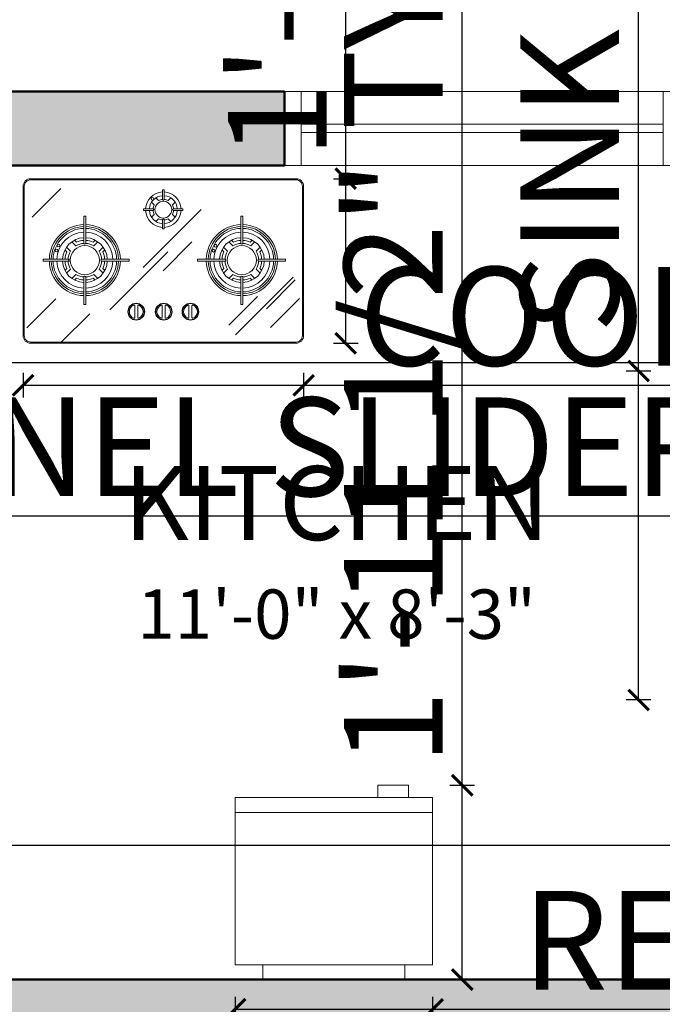
# Model space of a CAD drawing. Units: inches. Extents: x 375 to 1122, y 27 to 1069.
# Tile 152 of 155: x 819 to 897, y 872 to 991. Entities that reach past the tile are written whole.
import ezdxf

# ---------------------------------------------------------------- set-up
doc = ezdxf.new("R2010")
doc.units = ezdxf.units.IN
for name, color, linetype, lineweight in [('A-ANNO-DIMS', 2, 'Continuous', 18), ('A-AREA-IDEN', 7, 'Continuous', 18), ('A-EQPM', 55, 'Continuous', 18), ('A-FLOR-MILL', 55, 'Continuous', 25), ('A-WALL-PATT', 252, 'Continuous', 13), ('Walls', 250, 'Continuous', 50), ('Windows', 122, 'Continuous', 18)]:
    doc.layers.add(name, color=color, linetype=linetype, lineweight=lineweight)
doc.styles.get("Standard").update_dxf_attribs({"font": 'arial.ttf'})
doc.dimstyles.new('ISO-25', dxfattribs={"dimtxt": 12, "dimasz": 2.5, "dimexe": 1.5, "dimexo": 1.5, "dimtad": 1, "dimdec": 1, "dimlunit": 3, "dimtxsty": 'Standard', "dimblk": 'ARCHTICK', "dimcen": 2.5, "dimadec": 0, "dimazin": 0, "dimtfac": 1, "dimtdec": 1, "dimtmove": 0, "dimatfit": 3, "dimfxl": 1.5, "dimfxlon": 1, "dimarcsym": 0})

# ---------------------------------------------------------------- blocks, each defined once
blk = doc.blocks.new('A$C659B0DF6')
for p, q in [((17.35, 607.55), (17.35, 606.07)), ((21.05, 607.55), (17.35, 607.55)), ((21.05, 606.07), (21.05, 607.55)), ((24, 606.07), (0, 606.07)), ((0, 585.72), (0, 606.07)), ((24, 585.72), (24, 606.07)), ((24, 604.22), (0, 604.22)), ((24, 585.72), (0, 585.72)), ((3.37, 583.91), (3.37, 585.72)), ((20.63, 583.91), (20.63, 585.72)), ((3.37, 583.91), (20.63, 583.91))]:
    blk.add_line(p, q)
blk = doc.blocks.new('A$C038F079D')
for p, q in [((23.9, 336.8), (101.3, 414.2)), ((377.5, 410.6), (372.5, 410.6)), ((320.9, 202.7), (475.7, 357.5)), ((427.1, 359.8), (427.1, 354.8)), ((587.4, 339.9), (582.4, 339.9)), ((377.5, 305.6), (372.5, 305.6)), ((374.2, 193.8), (451.6, 271.2)), ((232.1, 89.3), (386.9, 244.1)), ((53.2, 224.7), (53.2, 219.7)), ((284, 224.7), (284, 219.7)), ((466, 224.7), (466, 219.7)), ((701.8, 224.7), (701.8, 219.7)), ((130.3, 173.3), (141.1, 184.1)), ((137.3, 169), (142.6, 174.2)), ((567.6, 22.2), (722.4, 177)), ((650.5, 92.2), (727.9, 169.6)), ((10.1, 41), (87.5, 118.4)), ((549.9, 47.9), (627.2, 125.3)), ((661.4, 42), (738.7, 119.3)), ((587.4, 103.7), (582.4, 103.7)), ((100.9, 1.5), (178.3, 78.9))]:
    blk.add_line(p, q)
at = {"ltscale": 0.18}
for p, q in [((372.5, 384.7), (372.5, 410.6)), ((377.5, 384.7), (377.5, 410.6)), ((350.8, 370.2), (343.5, 377.5)), ((362.2, 381.5), (354.8, 388.8)), ((387.8, 381.5), (395.2, 388.8)), ((399.2, 370.2), (406.5, 377.5)), ((322.3, 354.8), (322.3, 359.8)), ((347.6, 359.8), (322.3, 359.8)), ((347.6, 354.8), (322.3, 354.8)), ((343.5, 337.2), (350.8, 344.5)), ((406.5, 337.2), (399.2, 344.5)), ((402.4, 359.8), (427.1, 359.8)), ((402.4, 354.8), (427.1, 354.8)), ((162.6, 339.9), (167.6, 339.9)), ((162.6, 267.1), (162.6, 339.9)), ((167.6, 267.1), (167.6, 339.9)), ((354.8, 325.8), (362.2, 333.1)), ((372.5, 329.9), (372.5, 305.6)), ((377.5, 329.9), (377.5, 305.6)), ((395.2, 325.8), (387.8, 333.1)), ((582.4, 267.1), (582.4, 339.9)), ((587.4, 267.1), (587.4, 339.9)), ((130.3, 271.1), (141.1, 260.3)), ((137.3, 275.4), (142.6, 270.2)), ((187.6, 270.2), (192.8, 275.4)), ((189, 260.3), (199.8, 271.1)), ((561, 260.3), (550.2, 271.1)), ((562.4, 270.2), (557.2, 275.4)), ((612.7, 275.4), (607.4, 270.2)), ((619.7, 271.1), (608.9, 260.3)), ((111.9, 250), (117.1, 244.7)), ((116.2, 257), (127, 246.2)), ((203.2, 246.2), (214, 257)), ((213.1, 244.7), (218.3, 250)), ((536.9, 244.7), (531.7, 250)), ((546.8, 246.2), (536, 257)), ((633.8, 257), (623, 246.2)), ((638.1, 250), (632.9, 244.7)), ((125.1, 224.7), (53.2, 224.7)), ((125.1, 219.7), (53.2, 219.7)), ((210, 224.7), (284, 224.7)), ((210, 219.7), (284, 219.7)), ((540, 224.7), (466, 224.7)), ((540, 219.7), (466, 219.7)), ((629.9, 224.7), (701.8, 224.7)), ((629.9, 219.7), (701.8, 219.7)), ((111.9, 194.5), (117.1, 199.7)), ((116.2, 187.5), (127, 198.3)), ((203.2, 198.3), (214, 187.5)), ((213.1, 199.7), (218.3, 194.5)), ((536.9, 199.7), (531.7, 194.5)), ((546.8, 198.3), (536, 187.5)), ((633.8, 187.5), (623, 198.3)), ((638.1, 194.5), (632.9, 199.7)), ((162.6, 177.3), (162.6, 103.7)), ((167.6, 177.3), (167.6, 103.7)), ((187.6, 174.2), (192.8, 169)), ((189, 184.1), (199.8, 173.3)), ((561, 184.1), (550.2, 173.3)), ((562.4, 174.2), (557.2, 169)), ((582.4, 177.3), (582.4, 103.7)), ((587.4, 177.3), (587.4, 103.7)), ((612.7, 169), (607.4, 174.2)), ((619.7, 173.3), (608.9, 184.1)), ((162.6, 103.7), (167.6, 103.7)), ((298.6, 99.8), (298.6, 69)), ((306.6, 99.8), (306.6, 69)), ((372, 99.8), (372, 69)), ((380, 99.8), (380, 69)), ((443.4, 99.8), (443.4, 69)), ((451.4, 99.8), (451.4, 69))]:
    blk.add_line(p, q, dxfattribs=at)
for points in [[(20, 0), (730, 0, 0.414214), (750, 20), (750, 420, 0.414214), (730, 440), (20, 440, 0.414214), (0, 420), (0, 20, 0.414214)], [(20, 3), (730, 3, 0.414214), (747, 20), (747, 420, 0.414214), (730, 437), (20, 437, 0.414214), (3, 420), (3, 20, 0.414214)]]:
    blk.add_lwpolyline(points, format="xyb", close=True)
for centre in [(345.9, 386.3), (94.7, 261.5), (514.6, 260.8), (89.1, 248.3), (509, 247.6)]:
    blk.add_circle(centre, 3.73)
for centre, radius in [((375, 357.3), 22.4), ((165.1, 222.2), 39), ((584.9, 222.2), 39), ((302.6, 84.4), 22.5), ((302.6, 84.4), 21.5), ((376, 84.4), 22.5), ((376, 84.4), 21.5), ((447.4, 84.4), 22.5), ((447.4, 84.4), 21.5)]:
    blk.add_circle(centre, radius, dxfattribs=at)
for centre, radius, start, end in [((375, 357.3), 47.4, 93.0255, 176.9745), ((375, 357.3), 47.4, 3.0255, 86.9745), ((375, 357.3), 37.4, 93.8363, 176.1637), ((375, 357.3), 27.4, 151.9979, 174.8384), ((375, 357.3), 27.4, 95.203, 118.0021), ((375, 385), 2.52, 187.9505, 352.0495), ((375, 357.3), 37.4, 3.8363, 86.1637), ((375, 357.3), 27.4, 61.9979, 84.797), ((375, 357.3), 27.4, 5.206, 28.0021), ((375, 357.3), 47.4, 183.0255, 266.9745), ((375, 357.3), 37.4, 183.8363, 266.1637), ((346.8, 357.3), 2.62, 287.6318, 72.3682), ((375, 357.3), 27.4, 185.1616, 208.0021), ((375, 357.3), 47.4, 273.0255, 356.9745), ((375, 357.3), 37.4, 273.8363, 356.1637), ((375, 357.3), 27.4, 331.9979, 354.794), ((402.7, 357.3), 2.52, 97.2236, 262.7764), ((165.1, 222.2), 95, 91.5918, 178.4082), ((165.1, 222.2), 95, 1.5918, 88.4082), ((375, 357.3), 27.4, 241.9979, 264.7569), ((375, 330), 2.5, 358.3317, 181.6683), ((375, 357.3), 27.4, 275.2431, 298.0021), ((584.9, 222.2), 95, 91.5918, 178.4082), ((584.9, 222.2), 95, 1.5918, 88.4082), ((165.1, 222.2), 90, 91.5918, 178.4082), ((165.1, 222.2), 85, 91.6854, 178.3146), ((165.1, 222.2), 75, 91.9102, 178.0898), ((165.1, 222.2), 90, 1.5918, 88.4082), ((165.1, 222.2), 85, 1.6854, 88.3146), ((165.1, 222.2), 75, 1.9102, 88.0898), ((584.9, 222.2), 90, 91.5918, 178.4082), ((584.9, 222.2), 85, 91.6854, 178.3146), ((584.9, 222.2), 75, 91.9102, 178.0898), ((584.9, 222.2), 90, 1.5918, 88.4082), ((584.9, 222.2), 85, 1.6854, 88.3146), ((584.9, 222.2), 75, 1.9102, 88.0898), ((165.1, 222.2), 60, 92.388, 177.612), ((165.1, 222.2), 45, 93.1847, 122.1604), ((165.1, 222.2), 53, 92.7036, 115.1461), ((165.1, 267.4), 2.52, 186.7354, 353.2646), ((165.1, 222.2), 60, 2.388, 87.612), ((165.1, 222.2), 53, 64.8539, 87.2964), ((165.1, 222.2), 45, 57.8396, 86.8153), ((584.9, 222.2), 60, 92.388, 177.612), ((584.9, 222.2), 45, 93.1847, 122.1604), ((584.9, 222.2), 53, 92.7036, 115.1461), ((584.9, 267.3), 2.51, 183.9579, 356.0421), ((584.9, 222.2), 60, 2.388, 87.612), ((584.9, 222.2), 53, 64.8539, 87.2964), ((584.9, 222.2), 45, 57.8396, 86.8153), ((165.1, 222.2), 53, 154.8539, 177.2964), ((165.1, 222.2), 45, 147.8396, 176.8153), ((165.1, 222.2), 45, 3.1847, 32.1604), ((165.1, 222.2), 53, 2.7036, 25.1461), ((584.9, 222.2), 53, 154.8539, 177.2964), ((584.9, 222.2), 45, 147.8396, 176.8153), ((584.9, 222.2), 45, 3.1847, 32.1604), ((584.9, 222.2), 53, 2.7036, 25.1461), ((165.1, 222.2), 95, 181.5918, 268.4082), ((165.1, 222.2), 90, 181.5918, 268.4082), ((165.1, 222.2), 85, 181.6854, 268.3146), ((165.1, 222.2), 75, 181.9102, 268.0898), ((165.1, 222.2), 60, 182.388, 267.612), ((165.1, 222.2), 53, 182.7036, 205.1461), ((119.3, 222.2), 2.64, 288.751, 71.249), ((165.1, 222.2), 45, 183.1847, 212.1604), ((165.1, 222.2), 75, 271.9102, 358.0898), ((165.1, 222.2), 60, 272.388, 357.612), ((165.1, 222.2), 85, 271.6854, 358.3146), ((165.1, 222.2), 90, 271.5918, 358.4082), ((165.1, 222.2), 95, 271.5918, 358.4082), ((165.1, 222.2), 45, 327.8396, 356.8153), ((210.9, 222.2), 2.67, 110.5507, 249.4493), ((165.1, 222.2), 53, 334.8539, 357.2964), ((584.9, 222.2), 95, 181.5918, 268.4082), ((584.9, 222.2), 90, 181.5918, 268.4082), ((584.9, 222.2), 85, 181.6854, 268.3146), ((584.9, 222.2), 75, 181.9102, 268.0898), ((584.9, 222.2), 60, 182.388, 267.612), ((584.9, 222.2), 53, 182.7036, 205.1461), ((539.2, 222.2), 2.63, 288.412, 71.588), ((584.9, 222.2), 45, 183.1847, 212.1604), ((584.9, 222.2), 90, 271.5918, 358.4082), ((584.9, 222.2), 85, 271.6854, 358.3146), ((584.9, 222.2), 75, 271.9102, 358.0898), ((584.9, 222.2), 60, 272.388, 357.612), ((584.9, 222.2), 95, 271.5918, 358.4082), ((584.9, 222.2), 45, 327.8396, 356.8153), ((630.5, 222.2), 2.58, 104.2945, 255.7055), ((584.9, 222.2), 53, 334.8539, 357.2964), ((165.1, 222.2), 45, 237.8396, 266.8153), ((165.1, 222.2), 53, 244.8539, 267.2964), ((165.1, 222.2), 45, 273.1847, 302.1604), ((165.1, 222.2), 53, 272.7036, 295.1461), ((584.9, 222.2), 45, 237.8396, 266.8153), ((584.9, 222.2), 53, 244.8539, 267.2964), ((584.9, 176.5), 2.63, 17.9418, 162.0582), ((584.9, 222.2), 45, 273.1847, 302.1604), ((584.9, 222.2), 53, 272.7036, 295.1461), ((302.6, 84.4), 18.5, 111.3237, 248.6763), ((296.6, 99.8), 2, 0, 111.3237), ((308.6, 99.8), 2, 68.6763, 180), ((302.6, 84.4), 18.5, 291.3237, 68.6763), ((376, 84.4), 18.5, 111.3237, 248.6763), ((370, 99.8), 2, 0, 111.3237), ((382, 99.8), 2, 68.6763, 180), ((376, 84.4), 18.5, 291.3237, 68.6763), ((447.4, 84.4), 18.5, 111.3237, 248.6763), ((441.4, 99.8), 2, 0, 111.3237), ((453.4, 99.8), 2, 68.6763, 180), ((447.4, 84.4), 18.5, 291.3237, 68.6763), ((296.6, 69), 2, 248.6763, 0), ((308.6, 69), 2, 180, 291.3237), ((370, 69), 2, 248.6763, 0), ((382, 69), 2, 180, 291.3237), ((441.4, 69), 2, 248.6763, 0), ((453.4, 69), 2, 180, 291.3237)]:
    blk.add_arc(centre, radius, start, end, dxfattribs=at)
blk.add_arc((165.1, 176.3), 2.69, 21.7885, 158.2115)
blk = doc.blocks.new('_ArchTick')
at = {"color": 0, "linetype": 'ByBlock', "const_width": 0.15}
blk.add_lwpolyline([(-0.5, -0.5), (0.5, 0.5)], dxfattribs=at)
blk = doc.blocks.new('*D27')
at = {"layer": 'A-ANNO-DIMS', "color": 0, "lineweight": -2, "transparency": 16777216}
for p, q in [((444.51, 1030.21), (444.51, 1033.21)), ((986.01, 1030.21), (986.01, 1033.21)), ((444.51, 1031.71), (986.01, 1031.71))]:
    blk.add_line(p, q, dxfattribs=at)
at = {"layer": 'Defpoints', "color": 0, "transparency": 16777216}
for p in [(986.01, 1031.71), (444.51, 982.53), (986.01, 982.53)]:
    blk.add_point(p, dxfattribs=at)
at = {"layer": 'A-ANNO-DIMS', "color": 0, "lineweight": -2, "transparency": 16777216, "xscale": 2.5, "yscale": 2.5, "zscale": 2.5, "rotation": 180}
blk.add_blockref('_ArchTick', (444.51, 1031.71), dxfattribs=at)
at = {"layer": 'A-ANNO-DIMS', "color": 0, "lineweight": -2, "transparency": 16777216, "xscale": 2.5, "yscale": 2.5, "zscale": 2.5}
blk.add_blockref('_ArchTick', (986.01, 1031.71), dxfattribs=at)
at = {"layer": 'A-ANNO-DIMS', "color": 0, "transparency": 16777216, "insert": (715.26, 1038.46), "char_height": 12, "attachment_point": 5}
blk.add_mtext('45\'-1.5"', dxfattribs=at)
blk = doc.blocks.new('WINDOW-48IN')
for p, q in [((2, 5), (46, 5)), ((2, 4), (46, 4))]:
    blk.add_line(p, q)
blk.add_lwpolyline([(48, 0), (0, 0), (0, 9), (48, 9)], close=True)
for points in [[(2, 0), (2, 9)], [(46, 9), (46, 0)]]:
    blk.add_lwpolyline(points)
blk = doc.blocks.new('KITCHEN-COUNTER-L')
for p, q in [((0, 9), (0, 42)), ((87, 42), (0, 42)), ((87, 0), (87, 42)), ((87, 0), (111, 0))]:
    blk.add_line(p, q)
blk = doc.blocks.new('*D61')
at = {"layer": 'A-ANNO-DIMS', "color": 0, "lineweight": -2, "transparency": 16777216}
for p, q in [((845.01, 872.43), (845.01, 869.43)), ((869.01, 872.43), (869.01, 869.43)), ((845.01, 870.93), (869.01, 870.93)), ((869.01, 870.93), (1083.13, 870.93))]:
    blk.add_line(p, q, dxfattribs=at)
at = {"layer": 'Defpoints', "color": 0, "transparency": 16777216}
for p in [(845.01, 874.53), (869.01, 874.53), (869.01, 870.93)]:
    blk.add_point(p, dxfattribs=at)
at = {"layer": 'A-ANNO-DIMS', "color": 0, "lineweight": -2, "transparency": 16777216, "xscale": 2.5, "yscale": 2.5, "zscale": 2.5, "rotation": 180}
blk.add_blockref('_ArchTick', (845.01, 870.93), dxfattribs=at)
at = {"layer": 'A-ANNO-DIMS', "color": 0, "lineweight": -2, "transparency": 16777216, "xscale": 2.5, "yscale": 2.5, "zscale": 2.5}
blk.add_blockref('_ArchTick', (869.01, 870.93), dxfattribs=at)
at = {"layer": 'A-ANNO-DIMS', "color": 0, "transparency": 16777216, "insert": (977.32, 877.76), "char_height": 12, "attachment_point": 5}
blk.add_mtext('REFRIGERATOR 2\'-0" TYP.', dxfattribs=at)
blk = doc.blocks.new('*D62')
at = {"layer": 'A-ANNO-DIMS', "color": 0, "lineweight": -2, "transparency": 16777216}
for p, q in [((872.61, 898.16), (872.61, 1011.21)), ((871.11, 898.16), (874.11, 898.16)), ((872.61, 874.53), (872.61, 898.16)), ((871.11, 874.53), (874.11, 874.53))]:
    blk.add_line(p, q, dxfattribs=at)
at = {"layer": 'Defpoints', "color": 0, "transparency": 16777216}
for p in [(869.01, 898.16), (872.61, 898.16), (869.01, 874.53)]:
    blk.add_point(p, dxfattribs=at)
at = {"layer": 'A-ANNO-DIMS', "color": 0, "lineweight": -2, "transparency": 16777216, "xscale": 2.5, "yscale": 2.5, "zscale": 2.5}
for p, rotation in [((872.61, 898.16), 90), ((872.61, 874.53), 270)]:
    blk.add_blockref('_ArchTick', p, dxfattribs=dict(at, rotation=rotation))
at = {"layer": 'A-ANNO-DIMS', "color": 0, "transparency": 16777216, "insert": (865.78, 955.93), "char_height": 12, "attachment_point": 5, "rotation": 90}
blk.add_mtext('1\'-11 1/2" TYP.', dxfattribs=at)
blk = doc.blocks.new('*D63')
at = {"layer": 'A-ANNO-DIMS', "color": 0, "lineweight": -2, "transparency": 16777216}
for p, q in [((894.04, 948.53), (894.04, 1069.15)), ((895.54, 948.53), (892.54, 948.53)), ((894.04, 908.53), (894.04, 948.53)), ((895.54, 908.53), (892.54, 908.53))]:
    blk.add_line(p, q, dxfattribs=at)
at = {"layer": 'Defpoints', "color": 0, "transparency": 16777216}
for p in [(894.04, 948.53), (900.04, 948.53), (900.04, 908.53)]:
    blk.add_point(p, dxfattribs=at)
at = {"layer": 'A-ANNO-DIMS', "color": 0, "lineweight": -2, "transparency": 16777216, "xscale": 2.5, "yscale": 2.5, "zscale": 2.5}
for p, rotation in [((894.04, 948.53), 90), ((894.04, 908.53), 270)]:
    blk.add_blockref('_ArchTick', p, dxfattribs=dict(at, rotation=rotation))
at = {"layer": 'A-ANNO-DIMS', "color": 0, "transparency": 16777216, "insert": (887.21, 1010.09), "char_height": 12, "attachment_point": 5, "rotation": 90}
blk.add_mtext('SINK 3\'-4" TYP.', dxfattribs=at)
blk = doc.blocks.new('*D67')
at = {"layer": 'A-ANNO-DIMS', "color": 0, "lineweight": -2, "transparency": 16777216}
for p, q in [((819.23, 948.29), (819.23, 945.29)), ((853.33, 948.29), (853.33, 945.29)), ((819.23, 946.79), (853.33, 946.79)), ((853.33, 946.79), (1027.89, 946.79))]:
    blk.add_line(p, q, dxfattribs=at)
at = {"layer": 'Defpoints', "color": 0, "transparency": 16777216}
for p in [(819.23, 951.91), (853.33, 951.91), (853.33, 946.79)]:
    blk.add_point(p, dxfattribs=at)
at = {"layer": 'A-ANNO-DIMS', "color": 0, "lineweight": -2, "transparency": 16777216, "xscale": 2.5, "yscale": 2.5, "zscale": 2.5, "rotation": 180}
blk.add_blockref('_ArchTick', (819.23, 946.79), dxfattribs=at)
at = {"layer": 'A-ANNO-DIMS', "color": 0, "lineweight": -2, "transparency": 16777216, "xscale": 2.5, "yscale": 2.5, "zscale": 2.5}
blk.add_blockref('_ArchTick', (853.33, 946.79), dxfattribs=at)
at = {"layer": 'A-ANNO-DIMS', "color": 0, "transparency": 16777216, "insert": (941.86, 953.63), "char_height": 12, "attachment_point": 5}
blk.add_mtext('COOKTOP 2\'-10" TYP.', dxfattribs=at)
blk = doc.blocks.new('*D68')
at = {"layer": 'A-ANNO-DIMS', "color": 0, "lineweight": -2, "transparency": 16777216}
for p, q in [((858.44, 971.91), (858.44, 1047.67)), ((856.94, 971.91), (859.94, 971.91)), ((858.44, 951.91), (858.44, 971.91)), ((856.94, 951.91), (859.94, 951.91))]:
    blk.add_line(p, q, dxfattribs=at)
at = {"layer": 'Defpoints', "color": 0, "transparency": 16777216}
for p in [(853.33, 971.91), (858.44, 971.91), (853.33, 951.91)]:
    blk.add_point(p, dxfattribs=at)
at = {"layer": 'A-ANNO-DIMS', "color": 0, "lineweight": -2, "transparency": 16777216, "xscale": 2.5, "yscale": 2.5, "zscale": 2.5}
for p, rotation in [((858.44, 971.91), 90), ((858.44, 951.91), 270)]:
    blk.add_blockref('_ArchTick', p, dxfattribs=dict(at, rotation=rotation))
at = {"layer": 'A-ANNO-DIMS', "color": 0, "transparency": 16777216, "insert": (851.69, 1011.04), "char_height": 12, "attachment_point": 5, "rotation": 90}
blk.add_mtext('1\'-8" TYP.', dxfattribs=at)
blk = doc.blocks.new('*D73')
at = {"layer": 'A-ANNO-DIMS', "color": 0, "lineweight": -2, "transparency": 16777216}
for p, q in [((686.76, 932.43), (686.76, 929.43)), ((770.76, 932.43), (770.76, 929.43)), ((686.76, 930.93), (770.76, 930.93)), ((770.76, 930.93), (987.61, 930.93))]:
    blk.add_line(p, q, dxfattribs=at)
at = {"layer": 'Defpoints', "color": 0, "transparency": 16777216}
for p in [(686.76, 943.53), (770.76, 943.53), (770.76, 930.93)]:
    blk.add_point(p, dxfattribs=at)
at = {"layer": 'A-ANNO-DIMS', "color": 0, "lineweight": -2, "transparency": 16777216, "xscale": 2.5, "yscale": 2.5, "zscale": 2.5, "rotation": 180}
blk.add_blockref('_ArchTick', (686.76, 930.93), dxfattribs=at)
at = {"layer": 'A-ANNO-DIMS', "color": 0, "lineweight": -2, "transparency": 16777216, "xscale": 2.5, "yscale": 2.5, "zscale": 2.5}
blk.add_blockref('_ArchTick', (770.76, 930.93), dxfattribs=at)
at = {"layer": 'A-ANNO-DIMS', "color": 0, "transparency": 16777216, "insert": (880.43, 937.76), "char_height": 12, "attachment_point": 5}
blk.add_mtext('2-PANEL SLIDER 7\'-0" TYP.', dxfattribs=at)
blk = doc.blocks.new('*D77')
at = {"layer": 'A-ANNO-DIMS', "color": 0, "lineweight": -2, "transparency": 16777216}
for p, q in [((812.01, 892.38), (812.01, 889.38)), ((923.01, 892.38), (923.01, 889.38)), ((812.01, 890.88), (923.01, 890.88)), ((923.01, 890.88), (1101.82, 890.88))]:
    blk.add_line(p, q, dxfattribs=at)
at = {"layer": 'Defpoints', "color": 0, "transparency": 16777216}
for p in [(812.01, 907.53), (923.01, 907.53), (923.01, 890.88)]:
    blk.add_point(p, dxfattribs=at)
at = {"layer": 'A-ANNO-DIMS', "color": 0, "lineweight": -2, "transparency": 16777216, "xscale": 2.5, "yscale": 2.5, "zscale": 2.5, "rotation": 180}
blk.add_blockref('_ArchTick', (812.01, 890.88), dxfattribs=at)
at = {"layer": 'A-ANNO-DIMS', "color": 0, "lineweight": -2, "transparency": 16777216, "xscale": 2.5, "yscale": 2.5, "zscale": 2.5}
blk.add_blockref('_ArchTick', (923.01, 890.88), dxfattribs=at)
at = {"layer": 'A-ANNO-DIMS', "color": 0, "transparency": 16777216, "insert": (1013.66, 897.72), "char_height": 12, "attachment_point": 5}
blk.add_mtext('L-COUNTER 9\'-3" TYP.', dxfattribs=at)
blk = doc.blocks.new('*D88')
at = {"layer": 'A-ANNO-DIMS', "color": 0, "lineweight": -2, "transparency": 16777216}
for p, q in [((731.01, 1052.53), (731.01, 1055.53)), ((854.01, 1052.53), (854.01, 1055.53)), ((731.01, 1054.03), (854.01, 1054.03))]:
    blk.add_line(p, q, dxfattribs=at)
at = {"layer": 'Defpoints', "color": 0, "transparency": 16777216}
for p in [(854.01, 1054.03), (731.01, 502.53), (854.01, 502.53)]:
    blk.add_point(p, dxfattribs=at)
at = {"layer": 'A-ANNO-DIMS', "color": 0, "lineweight": -2, "transparency": 16777216, "xscale": 2.5, "yscale": 2.5, "zscale": 2.5, "rotation": 180}
blk.add_blockref('_ArchTick', (731.01, 1054.03), dxfattribs=at)
at = {"layer": 'A-ANNO-DIMS', "color": 0, "lineweight": -2, "transparency": 16777216, "xscale": 2.5, "yscale": 2.5, "zscale": 2.5}
blk.add_blockref('_ArchTick', (854.01, 1054.03), dxfattribs=at)
at = {"layer": 'A-ANNO-DIMS', "color": 0, "transparency": 16777216, "insert": (792.51, 1060.78), "char_height": 12, "attachment_point": 5}
blk.add_mtext('10\'-3"', dxfattribs=at)
blk = doc.blocks.new('*D96')
at = {"layer": 'A-ANNO-DIMS', "color": 0, "lineweight": -2, "transparency": 16777216}
for p, q in [((794.01, 1052.53), (794.01, 1055.53)), ((851.01, 1052.53), (851.01, 1055.53)), ((794.01, 1054.03), (851.01, 1054.03))]:
    blk.add_line(p, q, dxfattribs=at)
at = {"layer": 'Defpoints', "color": 0, "transparency": 16777216}
for p in [(851.01, 1054.03), (794.01, 973.53), (851.01, 973.53)]:
    blk.add_point(p, dxfattribs=at)
at = {"layer": 'A-ANNO-DIMS', "color": 0, "lineweight": -2, "transparency": 16777216, "xscale": 2.5, "yscale": 2.5, "zscale": 2.5, "rotation": 180}
blk.add_blockref('_ArchTick', (794.01, 1054.03), dxfattribs=at)
at = {"layer": 'A-ANNO-DIMS', "color": 0, "lineweight": -2, "transparency": 16777216, "xscale": 2.5, "yscale": 2.5, "zscale": 2.5}
blk.add_blockref('_ArchTick', (851.01, 1054.03), dxfattribs=at)
at = {"layer": 'A-ANNO-DIMS', "color": 0, "transparency": 16777216, "insert": (822.51, 1060.78), "char_height": 12, "attachment_point": 5}
blk.add_mtext('4\'-9"', dxfattribs=at)

msp = doc.modelspace()

# ---------------------------------------------------------------- hatches: boundary and pattern name
at = {"layer": 'A-WALL-PATT'}
h = msp.add_hatch(color=256, dxfattribs=at)
h.dxf.hatch_style = 1
h.paths.add_polyline_path([(962.01, 388.53), (989.01, 388.53), (989.01, 394.53), (962.01, 394.53), (932.01, 394.53), (932.01, 397.53), (923.01, 397.53), (923.01, 394.53), (842.01, 394.53), (842.01, 334.53), (839.51, 334.53), (839.51, 328.53), (854.01, 328.53), (854.01, 334.53), (848.01, 334.53), (848.01, 388.53), (953.01, 388.53), (953.01, 356.08), (962.01, 356.08), (962.01, 358.55), (989.01, 358.55), (989.01, 364.55), (962.01, 364.55)])
h.paths.add_polyline_path([(989.01, 502.53), (932.01, 502.53), (932.01, 583.53), (932.01, 593.53), (923.01, 593.53), (923.01, 583.53), (854.01, 583.53), (854.01, 556.53), (863.01, 556.53), (863.01, 574.53), (923.01, 574.53), (923.01, 502.53), (863.01, 502.53), (863.01, 520.53), (854.01, 520.53), (854.01, 502.53), (773.01, 502.53), (773.01, 493.53), (788.01, 493.53), (788.01, 402.03), (722.01, 402.03), (722.01, 373.53), (728.01, 373.53), (728.01, 396.03), (788.01, 396.03), (788.01, 373.53), (794.01, 373.53), (794.01, 430.53), (814.01, 430.53), (814.01, 436.53), (794.01, 436.53), (794.01, 493.53), (923.01, 493.53), (923.01, 487.53), (932.01, 487.53), (932.01, 493.53), (983.01, 493.53), (983.01, 473.53), (989.01, 473.53)])
h.paths.add_polyline_path([(797.01, 325.53), (805.01, 325.53), (805.01, 328.53), (807.51, 328.53), (807.51, 334.53), (791.01, 334.53), (791.01, 226.53), (770.76, 226.53), (770.76, 217.53), (791.01, 217.53), (791.01, 187.53), (855.01, 187.53), (855.01, 196.53), (797.01, 196.53)])
h.paths.add_polyline_path([(989.01, 238.53), (962.01, 238.53), (962.01, 256.42), (953.01, 256.42), (953.01, 229.53), (980.01, 229.53), (980.01, 196.53), (915.01, 196.53), (915.01, 187.53), (989.01, 187.53)])
h.paths.add_polyline_path([(962.01, 334.53), (884.01, 334.53), (884.01, 328.53), (918.01, 328.53), (918.01, 325.53), (932.01, 325.53), (932.01, 328.53), (953.01, 328.53), (953.01, 304.42), (962.01, 304.42)])
h.paths.add_polyline_path([(606.51, 283.53), (609.51, 283.53), (609.51, 289.53), (600.51, 289.53), (600.51, 196.53), (578.51, 196.53), (578.51, 187.53), (606.51, 187.53), (606.51, 196.53)])
h.paths.add_polyline_path([(666.51, 292.53), (660.51, 292.53), (660.51, 289.53), (633.51, 289.53), (633.51, 283.53), (660.51, 283.53), (660.51, 196.53), (628.01, 196.53), (628.01, 187.53), (630.53, 187.53), (630.53, 160.53), (636.53, 160.53), (636.53, 187.53), (660.51, 187.53), (660.51, 160.53), (666.51, 160.53), (666.51, 217.53), (686.76, 217.53), (686.76, 226.53), (666.51, 226.53)])
h.paths.add_polyline_path([(480.51, 256.42), (471.51, 256.42), (471.51, 238.53), (444.51, 238.53), (444.51, 187.53), (518.51, 187.53), (518.51, 196.53), (453.51, 196.53), (453.51, 229.53), (480.51, 229.53)])
h.paths.add_polyline_path([(480.51, 328.53), (652.51, 328.53), (652.51, 325.53), (660.51, 325.53), (660.51, 322.53), (666.51, 322.53), (666.51, 334.53), (507.51, 334.53), (507.51, 360.53), (498.51, 360.53), (498.51, 334.53), (471.51, 334.53), (471.51, 304.42), (480.51, 304.42)])
h.paths.add_polyline_path([(507.51, 484.53), (498.51, 484.53), (498.51, 444.53), (507.51, 444.53), (507.51, 454.53), (621.51, 454.53), (621.51, 460.53), (507.51, 460.53)])
h.paths.add_polyline_path([(672.51, 604.53), (683.26, 604.53), (683.26, 613.53), (669.51, 613.53), (669.51, 649.53), (663.51, 649.53), (663.51, 589.53), (507.51, 589.53), (507.51, 613.53), (498.51, 613.53), (498.51, 556.53), (507.51, 556.53), (507.51, 580.53), (663.51, 580.53), (663.51, 520.53), (669.51, 520.53), (669.51, 556.53), (683.26, 556.53), (683.26, 565.53), (672.51, 565.53)])
h.paths.add_polyline_path([(731.01, 667.53), (734.01, 667.53), (734.01, 676.53), (728.01, 676.53), (728.01, 715.53), (657.51, 715.53), (657.51, 709.53), (663.51, 709.53), (663.51, 673.53), (669.51, 673.53), (669.51, 709.53), (722.01, 709.53), (722.01, 613.53), (704.76, 613.53), (704.76, 604.53), (722.01, 604.53), (722.01, 565.53), (704.76, 565.53), (704.76, 556.53), (722.01, 556.53), (722.01, 502.53), (722.01, 460.53), (669.51, 460.53), (669.51, 496.53), (663.51, 496.53), (663.51, 460.53), (657.51, 460.53), (657.51, 454.53), (728.01, 454.53), (728.01, 493.53), (734.01, 493.53), (734.01, 502.53), (731.01, 502.53)])
h.paths.add_polyline_path([(986.01, 718.53), (959.01, 718.53), (959.01, 727.53), (950.01, 727.53), (950.01, 709.53), (977.01, 709.53), (977.01, 676.53), (794.01, 676.53), (794.01, 805.53), (802.01, 805.53), (802.01, 808.53), (804.51, 808.53), (804.51, 814.53), (788.01, 814.53), (788.01, 774.03), (728.01, 774.03), (728.01, 796.53), (722.01, 796.53), (722.01, 768.03), (788.01, 768.03), (788.01, 676.53), (773.01, 676.53), (773.01, 667.53), (923.01, 667.53), (923.01, 657.53), (932.01, 657.53), (932.01, 667.53), (986.01, 667.53)])
h.paths.add_polyline_path([(621.51, 715.53), (507.51, 715.53), (507.51, 733.53), (498.51, 733.53), (498.51, 715.53), (498.51, 685.53), (507.51, 685.53), (507.51, 709.53), (621.51, 709.53)])
h.paths.add_polyline_path([(666.51, 847.03), (660.51, 847.03), (660.51, 844.53), (652.51, 844.53), (652.51, 841.53), (480.51, 841.53), (480.51, 859.53), (471.51, 859.53), (471.51, 835.53), (498.51, 835.53), (498.51, 817.53), (507.51, 817.53), (507.51, 835.53), (666.51, 835.53)])
h.paths.add_polyline_path([(480.51, 940.53), (453.51, 940.53), (453.51, 973.53), (518.51, 973.53), (518.51, 982.53), (444.51, 982.53), (444.51, 931.53), (471.51, 931.53), (471.51, 907.53), (480.51, 907.53)])
h.paths.add_polyline_path([(606.51, 982.53), (578.51, 982.53), (578.51, 973.53), (600.51, 973.53), (600.51, 880.53), (609.51, 880.53), (609.51, 886.53), (606.51, 886.53)])
h.paths.add_polyline_path([(666.51, 943.53), (686.76, 943.53), (686.76, 952.53), (666.51, 952.53), (666.51, 1009.53), (660.51, 1009.53), (660.51, 982.53), (636.53, 982.53), (636.53, 1009.53), (630.53, 1009.53), (630.53, 982.53), (628.01, 982.53), (628.01, 973.53), (660.51, 973.53), (660.51, 886.53), (633.51, 886.53), (633.51, 880.53), (660.51, 880.53), (660.51, 877.03), (666.51, 877.03)])
h.paths.add_polyline_path([(986.01, 874.53), (932.01, 874.53), (932.01, 877.53), (923.01, 877.53), (923.01, 874.53), (788.01, 874.53), (788.01, 868.53), (788.01, 844.53), (794.01, 844.53), (794.01, 868.53), (839.01, 868.53), (839.01, 814.53), (836.51, 814.53), (836.51, 808.53), (851.01, 808.53), (851.01, 814.53), (845.01, 814.53), (845.01, 868.53), (986.01, 868.53)])
h.paths.add_polyline_path([(959.01, 838.55), (986.01, 838.55), (986.01, 844.55), (959.01, 844.55), (959.01, 847.03), (950.01, 847.03), (950.01, 814.53), (881.01, 814.53), (881.01, 808.53), (918.01, 808.53), (918.01, 805.53), (932.01, 805.53), (932.01, 808.53), (950.01, 808.53), (950.01, 793.53), (959.01, 793.53)])
h.paths.add_polyline_path([(986.01, 982.53), (899.01, 982.53), (899.01, 973.53), (923.01, 973.53), (923.01, 967.53), (932.01, 967.53), (932.01, 973.53), (980.01, 973.53), (980.01, 953.53), (986.01, 953.53)])
h.paths.add_polyline_path([(851.01, 982.53), (788.01, 982.53), (788.01, 952.53), (770.76, 952.53), (770.76, 943.53), (788.01, 943.53), (788.01, 910.53), (814.01, 910.53), (814.01, 916.53), (794.01, 916.53), (794.01, 973.53), (851.01, 973.53)])

# ---------------------------------------------------------------- linework, layer by layer
at = {"layer": 'Walls'}
for p, q in [((851.01, 982.53), (788.01, 982.53)), ((851.01, 973.53), (851.01, 982.53)), ((851.01, 973.53), (794.01, 973.53)), ((923.01, 874.53), (788.01, 874.53))]:
    msp.add_line(p, q, dxfattribs=at)

# ---------------------------------------------------------------- block references
at = {"layer": 'A-EQPM', "xscale": 0.0454545454545455, "yscale": 0.0454545454545455, "zscale": 0.0454545454545455}
msp.add_blockref('A$C038F079D', (819.23, 951.91), dxfattribs=at)
at = {"layer": 'A-EQPM'}
msp.add_blockref('A$C659B0DF6', (845.01, 290.61), dxfattribs=at)
at = {"layer": 'A-FLOR-MILL'}
msp.add_blockref('KITCHEN-COUNTER-L', (812.01, 907.53), dxfattribs=at)
at = {"layer": 'Windows'}
msp.add_blockref('WINDOW-48IN', (851.01, 973.53), dxfattribs=at)

# ---------------------------------------------------------------- texts
at = {"layer": 'A-AREA-IDEN', "insert": (824.28, 915.97), "char_height": 12, "attachment_point": 7}
msp.add_mtext_dynamic_manual_height_columns('\\pxqc;{\\fArial|b1|i0|c0|p34;\\H0.75x;KITCHEN\\H1.33333x;\\P\\fArial|b0|i0|c0|p34;\\H0.5x;11\'-0" x 8\'-3"}', width=66.1169, gutter_width=12.5, heights=[0], dxfattribs=at)

# ---------------------------------------------------------------- dimensions: what is measured, and where the dimension line sits
at = {"layer": 'A-ANNO-DIMS'}
for base, p1, p2, text, picture, middle in [((894.04, 948.53), (900.04, 908.53), (900.04, 948.53), 'SINK <> TYP.', '*D63', (887.21, 1010.09)), ((858.44, 971.91), (853.33, 951.91), (853.33, 971.91), '<> TYP.', '*D68', (851.69, 1011.04)), ((872.61, 898.16), (869.01, 874.53), (869.01, 898.16), '<> TYP.', '*D62', (865.78, 955.93))]:
    dim = msp.add_linear_dim(base=base, p1=p1, p2=p2, angle=90, text=text, dimstyle='ISO-25', override={"dimdec": 1, "dimlfac": 1, "dimrnd": 0, "dimzin": 1, "dimdsep": 46, "dimlunit": 4, "dimfrac": 2}, dxfattribs=at)
    dim.commit()
    dim.dimension.update_dxf_attribs({"geometry": picture, "text_midpoint": middle})
for base, p1, p2, picture, middle in [((854.01, 1054.03), (731.01, 502.53), (854.01, 502.53), '*D88', (792.51, 1060.78)), ((851.01, 1054.03), (794.01, 973.53), (851.01, 973.53), '*D96', (822.51, 1060.78))]:
    dim = msp.add_linear_dim(base=base, p1=p1, p2=p2, dimstyle='ISO-25', override={"dimdec": 1, "dimlfac": 1, "dimrnd": 0, "dimzin": 1, "dimdsep": 46, "dimlunit": 4, "dimfrac": 2}, dxfattribs=at)
    dim.commit()
    dim.dimension.update_dxf_attribs({"geometry": picture, "text_midpoint": middle})
dim = msp.add_linear_dim(base=(986.01, 1031.71), p1=(444.51, 982.53), p2=(986.01, 982.53), dimstyle='ISO-25', override={"dimclrd": 0, "dimclre": 0, "dimclrt": 0}, dxfattribs=at)
dim.commit()
dim.dimension.update_dxf_attribs({"geometry": '*D27', "text_midpoint": (715.26, 1031.71), "dimtype": 160})
for base, p1, p2, text, picture, middle in [((853.33, 946.79), (819.23, 951.91), (853.33, 951.91), 'COOKTOP <> TYP.', '*D67', (941.86, 953.63)), ((770.76, 930.93), (686.76, 943.53), (770.76, 943.53), '2-PANEL SLIDER <> TYP.', '*D73', (880.43, 937.76)), ((923.01, 890.88), (812.01, 907.53), (923.01, 907.53), 'L-COUNTER <> TYP.', '*D77', (1013.66, 897.72)), ((869.01, 870.93), (845.01, 874.53), (869.01, 874.53), 'REFRIGERATOR <> TYP.', '*D61', (977.32, 877.76))]:
    dim = msp.add_linear_dim(base=base, p1=p1, p2=p2, text=text, dimstyle='ISO-25', override={"dimdec": 1, "dimlfac": 1, "dimrnd": 0, "dimzin": 1, "dimdsep": 46, "dimlunit": 4, "dimfrac": 2}, dxfattribs=at)
    dim.commit()
    dim.dimension.update_dxf_attribs({"geometry": picture, "text_midpoint": middle})

doc.saveas('drawing.dxf')
